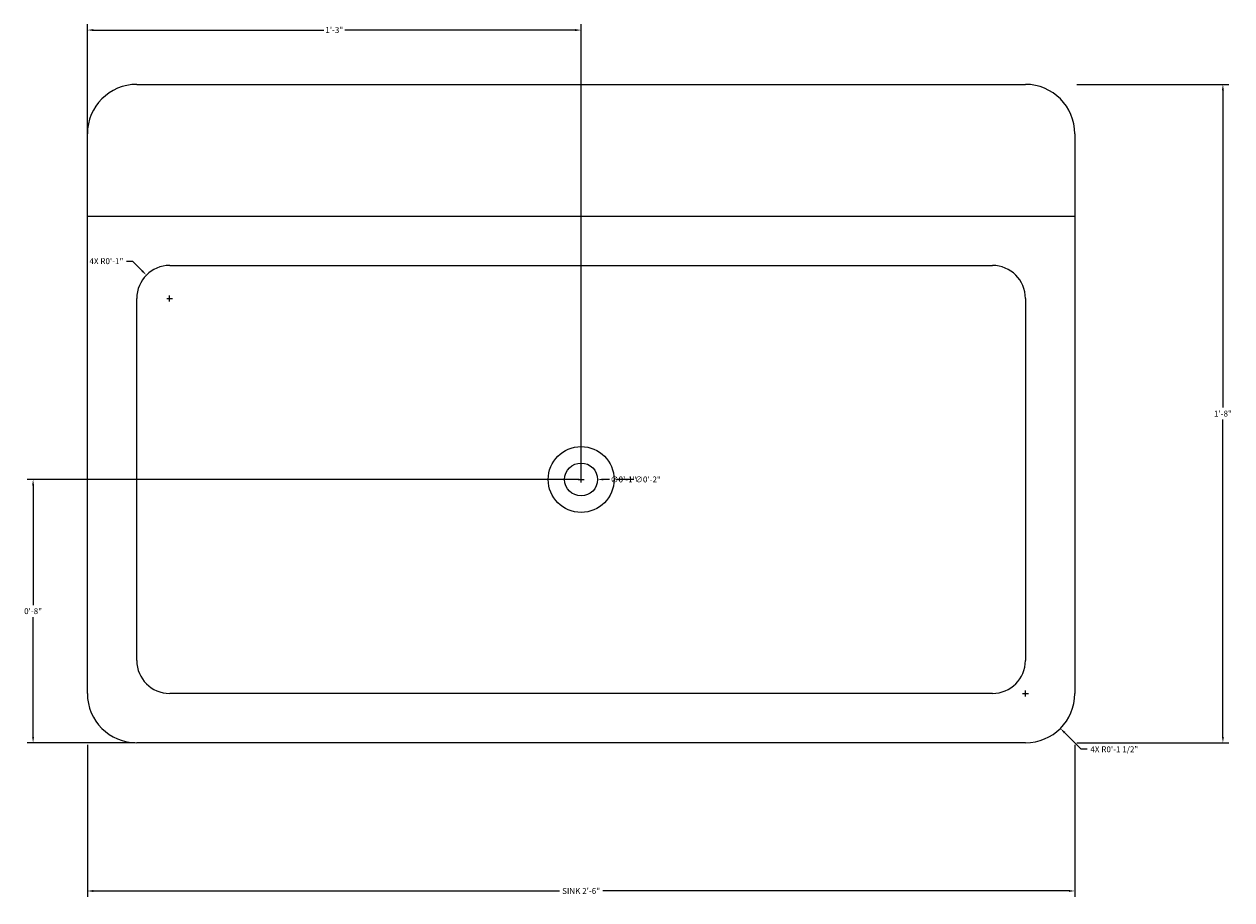
# Model space of a CAD drawing. Units: inches. Extents: x 226 to 1155, y 22 to 494.
# Tile 6 of 7: x 1118 to 1155, y 152 to 179. Entities that reach past the tile are written whole.
import ezdxf

# ---------------------------------------------------------------- set-up
doc = ezdxf.new("R2010")
doc.units = ezdxf.units.IN
doc.header["$MEASUREMENT"] = 0
doc.layers.add('A-ANNO-DIMS', color=2, linetype='Continuous', lineweight=18)
doc.layers.add('A-FLOR-FIXT', color=9, linetype='Continuous', lineweight=18)
doc.styles.get("Standard").update_dxf_attribs({"font": 'arial.ttf'})
doc.dimstyles.get("Standard").update_dxf_attribs({"dimtxt": 0.18, "dimasz": 0.18, "dimexe": 0.18, "dimexo": 0.0625, "dimgap": 0.09, "dimtad": 0, "dimtih": 1, "dimtoh": 1, "dimdec": 4, "dimzin": 0, "dimdsep": 46, "dimlunit": 4, "dimtxsty": 'Standard', "dimcen": 0.09, "dimadec": 0, "dimazin": 0, "dimtfac": 1, "dimtdec": 4, "dimtofl": 0, "dimtmove": 0, "dimatfit": 3, "dimfxl": 1, "dimtolj": 1, "dimtzin": 0, "dimarcsym": 0})

# ---------------------------------------------------------------- blocks, each defined once
blk = doc.blocks.new('Sink-single - 30 in top')
blk.add_line((-15, -3.999996), (15, -3.999996))
for points in [[(-13.5, 0), (13.5, 0)], [(-15, -18.499996), (-15, -1.5)], [(15, -1.5), (15, -18.499996)], [(-12.5, -5.499996), (12.5, -5.499996)], [(-13.5, -17.499996), (-13.5, -6.499996)], [(13.5, -6.499996), (13.5, -17.499996)], [(12.5, -18.499996), (-12.5, -18.499996)], [(13.5, -19.999996), (-13.5, -19.999996)]]:
    blk.add_lwpolyline(points)
for radius in [1, 0.5]:
    blk.add_circle((0, -11.999996), radius)
for centre, radius, start, end in [((-13.5, -1.5), 1.5, 90, 180), ((13.5, -1.5), 1.5, 0, 90), ((-12.5, -6.499996), 1, 90, 180), ((12.5, -6.499996), 1, 0, 90), ((-12.5, -17.499996), 1, 180, 270), ((12.5, -17.499996), 1, 270, 0), ((-13.5, -18.499996), 1.5, 180, 270), ((13.5, -18.499996), 1.5, 270, 0)]:
    blk.add_arc(centre, radius, start, end)
blk = doc.blocks.new('*D50')
at = {"layer": 'A-ANNO-DIMS', "color": 0, "lineweight": -2, "transparency": 16777216}
for p, q in [((1120.169, 156.868), (1120.169, 152.251)), ((1150.169, 156.868), (1150.169, 152.251)), ((1120.349, 152.431), (1134.512, 152.431)), ((1149.989, 152.431), (1135.827, 152.431))]:
    blk.add_line(p, q, dxfattribs=at)
at = {"layer": 'A-ANNO-DIMS', "color": 0, "transparency": 16777216}
for points in [[(1120.349, 152.461), (1120.349, 152.401), (1120.169, 152.431)], [(1149.989, 152.461), (1149.989, 152.401), (1150.169, 152.431)]]:
    blk.add_solid(points, dxfattribs=at)
at = {"layer": 'Defpoints', "color": 0, "transparency": 16777216}
for p in [(1120.169, 156.931), (1150.169, 156.931), (1150.169, 152.431)]:
    blk.add_point(p, dxfattribs=at)
at = {"layer": 'A-ANNO-DIMS', "color": 0, "transparency": 16777216, "insert": (1135.169, 152.431), "char_height": 0.18, "attachment_point": 5}
blk.add_mtext('\\A1;SINK 2\'-6"', dxfattribs=at)
blk = doc.blocks.new('*D51')
at = {"layer": 'A-ANNO-DIMS', "color": 0, "lineweight": -2, "transparency": 16777216}
for p, q in [((1150.232, 176.931), (1154.849, 176.931)), ((1154.669, 176.751), (1154.669, 167.112)), ((1154.669, 157.111), (1154.669, 166.749)), ((1150.232, 156.931), (1154.849, 156.931))]:
    blk.add_line(p, q, dxfattribs=at)
at = {"layer": 'A-ANNO-DIMS', "color": 0, "transparency": 16777216}
for points in [[(1154.639, 176.751), (1154.699, 176.751), (1154.669, 176.931)], [(1154.639, 157.111), (1154.699, 157.111), (1154.669, 156.931)]]:
    blk.add_solid(points, dxfattribs=at)
at = {"layer": 'Defpoints', "color": 0, "transparency": 16777216}
for p in [(1150.169, 176.931), (1154.669, 176.931), (1150.169, 156.931)]:
    blk.add_point(p, dxfattribs=at)
at = {"layer": 'A-ANNO-DIMS', "color": 0, "transparency": 16777216, "insert": (1154.669, 166.931), "char_height": 0.18, "attachment_point": 5}
blk.add_mtext('\\A1;1\'-8"', dxfattribs=at)
blk = doc.blocks.new('*D102')
at = {"layer": 'A-ANNO-DIMS', "color": 0, "lineweight": -2, "transparency": 16777216}
for p, q in [((1120.169, 158.493), (1120.169, 178.761)), ((1135.169, 164.993), (1135.169, 178.761)), ((1120.349, 178.581), (1127.349, 178.581)), ((1134.989, 178.581), (1127.99, 178.581))]:
    blk.add_line(p, q, dxfattribs=at)
at = {"layer": 'A-ANNO-DIMS', "color": 0, "transparency": 16777216}
for points in [[(1120.349, 178.611), (1120.349, 178.551), (1120.169, 178.581)], [(1134.989, 178.611), (1134.989, 178.551), (1135.169, 178.581)]]:
    blk.add_solid(points, dxfattribs=at)
at = {"layer": 'Defpoints', "color": 0, "transparency": 16777216}
for p in [(1135.169, 178.581), (1135.169, 164.931), (1120.169, 158.431)]:
    blk.add_point(p, dxfattribs=at)
at = {"layer": 'A-ANNO-DIMS', "color": 0, "transparency": 16777216, "insert": (1127.669, 178.581), "char_height": 0.18, "attachment_point": 5}
blk.add_mtext('\\A1;1\'-3"', dxfattribs=at)
blk = doc.blocks.new('*D103')
at = {"layer": 'A-ANNO-DIMS', "color": 0, "lineweight": -2, "transparency": 16777216}
for p, q in [((1135.107, 164.931), (1118.339, 164.931)), ((1118.519, 164.751), (1118.519, 161.112)), ((1118.519, 157.111), (1118.519, 160.749)), ((1121.607, 156.931), (1118.339, 156.931))]:
    blk.add_line(p, q, dxfattribs=at)
at = {"layer": 'A-ANNO-DIMS', "color": 0, "transparency": 16777216}
for points in [[(1118.489, 164.751), (1118.549, 164.751), (1118.519, 164.931)], [(1118.489, 157.111), (1118.549, 157.111), (1118.519, 156.931)]]:
    blk.add_solid(points, dxfattribs=at)
at = {"layer": 'Defpoints', "color": 0, "transparency": 16777216}
for p in [(1118.519, 164.931), (1135.169, 164.931), (1121.669, 156.931)]:
    blk.add_point(p, dxfattribs=at)
at = {"layer": 'A-ANNO-DIMS', "color": 0, "transparency": 16777216, "insert": (1118.519, 160.931), "char_height": 0.18, "attachment_point": 5}
blk.add_mtext('\\A1;0\'-8"', dxfattribs=at)
blk = doc.blocks.new('*D123')
at = {"layer": 'A-ANNO-DIMS', "color": 0, "lineweight": -2, "transparency": 16777216}
for p, q in [((1148.669, 158.341), (1148.669, 158.521)), ((1148.579, 158.431), (1148.759, 158.431)), ((1150.366, 156.734), (1149.857, 157.243)), ((1150.546, 156.734), (1150.366, 156.734))]:
    blk.add_line(p, q, dxfattribs=at)
at = {"layer": 'A-ANNO-DIMS', "color": 0, "transparency": 16777216}
blk.add_solid([(1149.879, 157.264), (1149.836, 157.221), (1149.73, 157.37)], dxfattribs=at)
at = {"layer": 'Defpoints', "color": 0, "transparency": 16777216}
for p in [(1148.669, 158.431), (1149.73, 157.37)]:
    blk.add_point(p, dxfattribs=at)
at = {"layer": 'A-ANNO-DIMS', "color": 0, "transparency": 16777216, "insert": (1151.369, 156.734), "char_height": 0.18, "attachment_point": 5}
blk.add_mtext('\\A1;4X R0\'-1 1/2"', dxfattribs=at)
blk = doc.blocks.new('*D124')
at = {"layer": 'A-ANNO-DIMS', "color": 0, "lineweight": -2, "transparency": 16777216}
for p, q in [((1121.358, 171.562), (1121.538, 171.562)), ((1121.538, 171.562), (1121.835, 171.265)), ((1122.579, 170.431), (1122.759, 170.431)), ((1122.669, 170.341), (1122.669, 170.521))]:
    blk.add_line(p, q, dxfattribs=at)
at = {"layer": 'A-ANNO-DIMS', "color": 0, "transparency": 16777216}
blk.add_solid([(1121.856, 171.286), (1121.814, 171.244), (1121.962, 171.138)], dxfattribs=at)
at = {"layer": 'Defpoints', "color": 0, "transparency": 16777216}
for p in [(1121.962, 171.138), (1122.669, 170.431)]:
    blk.add_point(p, dxfattribs=at)
at = {"layer": 'A-ANNO-DIMS', "color": 0, "transparency": 16777216, "insert": (1120.746, 171.562), "char_height": 0.18, "attachment_point": 5}
blk.add_mtext('\\A1;4X R0\'-1"', dxfattribs=at)
blk = doc.blocks.new('*D125')
at = {"layer": 'A-ANNO-DIMS', "color": 0, "lineweight": -2, "transparency": 16777216}
for p, q in [((1135.079, 164.931), (1135.259, 164.931)), ((1135.169, 164.841), (1135.169, 165.021)), ((1136.769, 164.931), (1136.349, 164.931))]:
    blk.add_line(p, q, dxfattribs=at)
at = {"layer": 'A-ANNO-DIMS', "color": 0, "transparency": 16777216}
blk.add_solid([(1136.349, 164.961), (1136.349, 164.901), (1136.169, 164.931)], dxfattribs=at)
at = {"layer": 'Defpoints', "color": 0, "transparency": 16777216}
for p in [(1134.169, 164.93), (1136.169, 164.931)]:
    blk.add_point(p, dxfattribs=at)
at = {"layer": 'A-ANNO-DIMS', "color": 0, "transparency": 16777216, "insert": (1137.197, 164.931), "char_height": 0.18, "attachment_point": 5}
blk.add_mtext('\\A1;∅0\'-2"', dxfattribs=at)
blk = doc.blocks.new('*D126')
at = {"layer": 'A-ANNO-DIMS', "color": 0, "lineweight": -2, "transparency": 16777216}
for p, q in [((1135.079, 164.931), (1135.259, 164.931)), ((1135.169, 164.841), (1135.169, 165.021)), ((1136.029, 164.931), (1135.849, 164.931))]:
    blk.add_line(p, q, dxfattribs=at)
at = {"layer": 'A-ANNO-DIMS', "color": 0, "transparency": 16777216}
blk.add_solid([(1135.849, 164.961), (1135.849, 164.901), (1135.669, 164.931)], dxfattribs=at)
at = {"layer": 'Defpoints', "color": 0, "transparency": 16777216}
for p in [(1134.669, 164.93), (1135.669, 164.931)]:
    blk.add_point(p, dxfattribs=at)
at = {"layer": 'A-ANNO-DIMS', "color": 0, "transparency": 16777216, "insert": (1136.457, 164.931), "char_height": 0.18, "attachment_point": 5}
blk.add_mtext('\\A1;∅0\'-1"', dxfattribs=at)

msp = doc.modelspace()

# ---------------------------------------------------------------- block references
at = {"layer": 'A-FLOR-FIXT'}
msp.add_blockref('Sink-single - 30 in top', (1135.16941, 176.93058), dxfattribs=at)

# ---------------------------------------------------------------- dimensions: what is measured, and where the dimension line sits
at = {"layer": 'A-ANNO-DIMS'}
dim = msp.add_linear_dim(base=(1135.16941, 178.58058), p1=(1120.16941, 158.43058), p2=(1135.16941, 164.93058), dimstyle='Standard', override={"dimdec": 1, "dimlfac": 1, "dimrnd": 0, "dimzin": 1, "dimdsep": 46, "dimlunit": 4, "dimfrac": 2}, dxfattribs=at)
dim.commit()
dim.dimension.update_dxf_attribs({"geometry": '*D102', "text_midpoint": (1127.66941, 178.58058)})
for base, p1, p2, picture, middle in [((1154.66941, 176.93058), (1150.16941, 156.93058), (1150.16941, 176.93058), '*D51', (1154.66941, 166.93058)), ((1118.51941, 164.93058), (1121.66941, 156.93058), (1135.16941, 164.93058), '*D103', (1118.51941, 160.93058))]:
    dim = msp.add_linear_dim(base=base, p1=p1, p2=p2, angle=90, dimstyle='Standard', override={"dimdec": 1, "dimlfac": 1, "dimrnd": 0, "dimzin": 1, "dimdsep": 46, "dimlunit": 4, "dimfrac": 2}, dxfattribs=at)
    dim.commit()
    dim.dimension.update_dxf_attribs({"geometry": picture, "text_midpoint": middle})
for center, mpoint, picture, middle in [((1122.66941, 170.43058), (1121.96231, 171.13769), '*D124', (1120.74567, 171.56196)), ((1148.66941, 158.43058), (1149.73007, 157.36993), '*D123', (1151.36857, 156.73353))]:
    dim = msp.add_radius_dim(center=center, mpoint=mpoint, text='4X <>', dimstyle='Standard', override={"dimdec": 1, "dimlfac": 1, "dimrnd": 0, "dimzin": 1, "dimdsep": 46, "dimlunit": 4, "dimfrac": 2}, dxfattribs=at)
    dim.commit()
    dim.dimension.update_dxf_attribs({"geometry": picture, "text_midpoint": middle, "dimtype": 164})
dim = msp.add_diameter_dim_2p(p1=(1134.16941, 164.93016), p2=(1136.16941, 164.931), dimstyle='Standard', override={"dimdec": 1, "dimlfac": 1, "dimrnd": 0, "dimzin": 1, "dimdsep": 46, "dimlunit": 4, "dimfrac": 2}, dxfattribs=at)
dim.commit()
dim.dimension.update_dxf_attribs({"geometry": '*D125', "text_midpoint": (1136.76941, 164.93125), "dimtype": 163})
dim = msp.add_diameter_dim_2p(p1=(1134.66941, 164.93016), p2=(1135.66941, 164.931), dimstyle='Standard', override={"dimdec": 1, "dimlfac": 1, "dimrnd": 0, "dimzin": 1, "dimdsep": 46, "dimlunit": 4, "dimfrac": 2}, dxfattribs=at)
dim.commit()
dim.dimension.update_dxf_attribs({"geometry": '*D126', "text_midpoint": (1136.02941, 164.9313)})
dim = msp.add_linear_dim(base=(1150.16941, 152.43058), p1=(1120.16941, 156.93058), p2=(1150.16941, 156.93058), text='SINK <>', dimstyle='Standard', override={"dimdec": 1, "dimlfac": 1, "dimrnd": 0, "dimzin": 1, "dimdsep": 46, "dimlunit": 4, "dimfrac": 2}, dxfattribs=at)
dim.commit()
dim.dimension.update_dxf_attribs({"geometry": '*D50', "text_midpoint": (1135.16941, 152.43058)})

doc.saveas('drawing.dxf')
